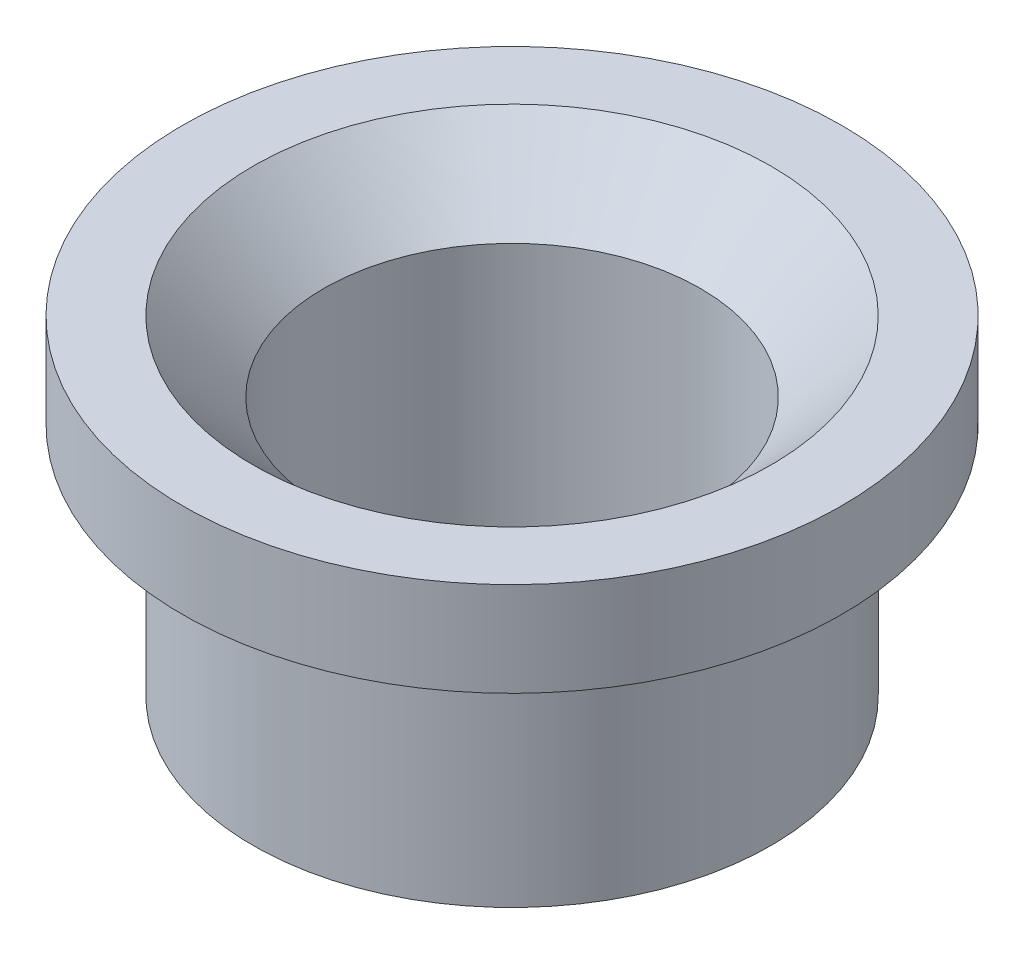
ISO-10303-21;
HEADER;
FILE_DESCRIPTION(('STEP AP214'),'2;1');
FILE_NAME('part.step','',(''),(''),'','','');
FILE_SCHEMA(('AUTOMOTIVE_DESIGN { 1 0 10303 214 1 1 1 1 }'));
ENDSEC;
DATA;
#1=APPLICATION_CONTEXT('core data for automotive mechanical design processes');
#2=APPLICATION_PROTOCOL_DEFINITION('international standard','automotive_design',2000,#1);
#3=PRODUCT_CONTEXT('',#1,'mechanical');
#4=PRODUCT('Part','Part','',(#3));
#5=PRODUCT_RELATED_PRODUCT_CATEGORY('part','',(#4));
#6=PRODUCT_DEFINITION_FORMATION('','',#4);
#7=PRODUCT_DEFINITION_CONTEXT('part definition',#1,'design');
#8=PRODUCT_DEFINITION('design','',#6,#7);
#9=PRODUCT_DEFINITION_SHAPE('','',#8);
#10=(LENGTH_UNIT() NAMED_UNIT(*) SI_UNIT(.MILLI.,.METRE.));
#11=(NAMED_UNIT(*) PLANE_ANGLE_UNIT() SI_UNIT($,.RADIAN.));
#12=(NAMED_UNIT(*) SI_UNIT($,.STERADIAN.) SOLID_ANGLE_UNIT());
#13=UNCERTAINTY_MEASURE_WITH_UNIT(LENGTH_MEASURE(1.E-05),#10,'distance_accuracy_value','');
#14=(GEOMETRIC_REPRESENTATION_CONTEXT(3) GLOBAL_UNCERTAINTY_ASSIGNED_CONTEXT((#13)) GLOBAL_UNIT_ASSIGNED_CONTEXT((#10,
#11,#12)) REPRESENTATION_CONTEXT('',''));
#15=CARTESIAN_POINT('',(0.,0.,0.));
#16=DIRECTION('',(0.,0.,1.));
#17=DIRECTION('',(1.,0.,0.));
#18=AXIS2_PLACEMENT_3D('',#15,#16,#17);
#19=CARTESIAN_POINT('',(16.5,0.,0.));
#20=DIRECTION('',(0.,-1.,0.));
#21=DIRECTION('',(0.,0.,-1.));
#22=AXIS2_PLACEMENT_3D('',#19,#20,#21);
#23=PLANE('',#22);
#24=CARTESIAN_POINT('',(0.,0.,0.));
#25=DIRECTION('',(0.,-1.,0.));
#26=DIRECTION('',(0.,0.,-1.));
#27=AXIS2_PLACEMENT_3D('',#24,#25,#26);
#28=CIRCLE('',#27,16.5);
#29=CARTESIAN_POINT('',(0.,0.,-16.5));
#30=VERTEX_POINT('',#29);
#31=EDGE_CURVE('E65',#30,#30,#28,.T.);
#32=ORIENTED_EDGE('',*,*,#31,.T.);
#33=EDGE_LOOP('',(#32));
#34=FACE_BOUND('',#33,.T.);
#35=CARTESIAN_POINT('',(0.,0.,0.));
#36=DIRECTION('',(0.,-1.,0.));
#37=DIRECTION('',(0.,0.,-1.));
#38=AXIS2_PLACEMENT_3D('',#35,#36,#37);
#39=CIRCLE('',#38,12.);
#40=CARTESIAN_POINT('',(0.,0.,-12.));
#41=VERTEX_POINT('',#40);
#42=EDGE_CURVE('E10',#41,#41,#39,.T.);
#43=ORIENTED_EDGE('',*,*,#42,.F.);
#44=EDGE_LOOP('',(#43));
#45=FACE_BOUND('',#44,.T.);
#46=ADVANCED_FACE('F40',(#34,#45),#23,.T.);
#47=CARTESIAN_POINT('',(0.,0.,0.));
#48=DIRECTION('',(0.,-1.,0.));
#49=DIRECTION('',(0.,0.,-1.));
#50=AXIS2_PLACEMENT_3D('',#47,#48,#49);
#51=CYLINDRICAL_SURFACE('',#50,12.);
#52=ORIENTED_EDGE('',*,*,#42,.T.);
#53=EDGE_LOOP('',(#52));
#54=FACE_BOUND('',#53,.T.);
#55=CARTESIAN_POINT('',(0.,16.5,0.));
#56=DIRECTION('',(0.,-1.,0.));
#57=DIRECTION('',(0.,0.,-1.));
#58=AXIS2_PLACEMENT_3D('',#55,#56,#57);
#59=CIRCLE('',#58,12.);
#60=CARTESIAN_POINT('',(0.,16.5,-12.));
#61=VERTEX_POINT('',#60);
#62=EDGE_CURVE('E43',#61,#61,#59,.T.);
#63=ORIENTED_EDGE('',*,*,#62,.F.);
#64=EDGE_LOOP('',(#63));
#65=FACE_BOUND('',#64,.T.);
#66=ADVANCED_FACE('F78',(#54,#65),#51,.F.);
#67=CARTESIAN_POINT('',(0.,21.,0.));
#68=DIRECTION('',(0.,1.,0.));
#69=DIRECTION('',(0.,0.,1.));
#70=AXIS2_PLACEMENT_3D('',#67,#68,#69);
#71=CONICAL_SURFACE('',#70,16.5,0.785398163397446);
#72=ORIENTED_EDGE('',*,*,#62,.T.);
#73=EDGE_LOOP('',(#72));
#74=FACE_BOUND('',#73,.T.);
#75=CARTESIAN_POINT('',(0.,21.,0.));
#76=DIRECTION('',(0.,-1.,0.));
#77=DIRECTION('',(0.,0.,-1.));
#78=AXIS2_PLACEMENT_3D('',#75,#76,#77);
#79=CIRCLE('',#78,16.5);
#80=CARTESIAN_POINT('',(0.,21.,-16.5));
#81=VERTEX_POINT('',#80);
#82=EDGE_CURVE('E50',#81,#81,#79,.T.);
#83=ORIENTED_EDGE('',*,*,#82,.F.);
#84=EDGE_LOOP('',(#83));
#85=FACE_BOUND('',#84,.T.);
#86=ADVANCED_FACE('F83',(#74,#85),#71,.F.);
#87=CARTESIAN_POINT('',(16.5,21.,0.));
#88=DIRECTION('',(0.,1.,0.));
#89=DIRECTION('',(0.,0.,1.));
#90=AXIS2_PLACEMENT_3D('',#87,#88,#89);
#91=PLANE('',#90);
#92=ORIENTED_EDGE('',*,*,#82,.T.);
#93=EDGE_LOOP('',(#92));
#94=FACE_BOUND('',#93,.T.);
#95=CARTESIAN_POINT('',(0.,21.,0.));
#96=DIRECTION('',(0.,-1.,0.));
#97=DIRECTION('',(0.,0.,-1.));
#98=AXIS2_PLACEMENT_3D('',#95,#96,#97);
#99=CIRCLE('',#98,21.);
#100=CARTESIAN_POINT('',(0.,21.,-21.));
#101=VERTEX_POINT('',#100);
#102=EDGE_CURVE('E51',#101,#101,#99,.T.);
#103=ORIENTED_EDGE('',*,*,#102,.F.);
#104=EDGE_LOOP('',(#103));
#105=FACE_BOUND('',#104,.T.);
#106=ADVANCED_FACE('F86',(#94,#105),#91,.T.);
#107=CARTESIAN_POINT('',(0.,0.,0.));
#108=DIRECTION('',(0.,-1.,0.));
#109=DIRECTION('',(0.,0.,-1.));
#110=AXIS2_PLACEMENT_3D('',#107,#108,#109);
#111=CYLINDRICAL_SURFACE('',#110,21.);
#112=ORIENTED_EDGE('',*,*,#102,.T.);
#113=EDGE_LOOP('',(#112));
#114=FACE_BOUND('',#113,.T.);
#115=CARTESIAN_POINT('',(0.,15.,0.));
#116=DIRECTION('',(0.,-1.,0.));
#117=DIRECTION('',(0.,0.,-1.));
#118=AXIS2_PLACEMENT_3D('',#115,#116,#117);
#119=CIRCLE('',#118,21.);
#120=CARTESIAN_POINT('',(0.,15.,-21.));
#121=VERTEX_POINT('',#120);
#122=EDGE_CURVE('E57',#121,#121,#119,.T.);
#123=ORIENTED_EDGE('',*,*,#122,.F.);
#124=EDGE_LOOP('',(#123));
#125=FACE_BOUND('',#124,.T.);
#126=ADVANCED_FACE('F77',(#114,#125),#111,.T.);
#127=CARTESIAN_POINT('',(21.,15.,0.));
#128=DIRECTION('',(0.,-1.,0.));
#129=DIRECTION('',(0.,0.,-1.));
#130=AXIS2_PLACEMENT_3D('',#127,#128,#129);
#131=PLANE('',#130);
#132=ORIENTED_EDGE('',*,*,#122,.T.);
#133=EDGE_LOOP('',(#132));
#134=FACE_BOUND('',#133,.T.);
#135=CARTESIAN_POINT('',(0.,15.,0.));
#136=DIRECTION('',(0.,-1.,0.));
#137=DIRECTION('',(0.,0.,-1.));
#138=AXIS2_PLACEMENT_3D('',#135,#136,#137);
#139=CIRCLE('',#138,16.5);
#140=CARTESIAN_POINT('',(0.,15.,-16.5));
#141=VERTEX_POINT('',#140);
#142=EDGE_CURVE('E56',#141,#141,#139,.T.);
#143=ORIENTED_EDGE('',*,*,#142,.F.);
#144=EDGE_LOOP('',(#143));
#145=FACE_BOUND('',#144,.T.);
#146=ADVANCED_FACE('F70',(#134,#145),#131,.T.);
#147=CARTESIAN_POINT('',(0.,0.,0.));
#148=DIRECTION('',(0.,-1.,0.));
#149=DIRECTION('',(0.,0.,-1.));
#150=AXIS2_PLACEMENT_3D('',#147,#148,#149);
#151=CYLINDRICAL_SURFACE('',#150,16.5);
#152=ORIENTED_EDGE('',*,*,#142,.T.);
#153=EDGE_LOOP('',(#152));
#154=FACE_BOUND('',#153,.T.);
#155=ORIENTED_EDGE('',*,*,#31,.F.);
#156=EDGE_LOOP('',(#155));
#157=FACE_BOUND('',#156,.T.);
#158=ADVANCED_FACE('F69',(#154,#157),#151,.T.);
#159=CLOSED_SHELL('',(#46,#66,#86,#106,#126,#146,#158));
#160=MANIFOLD_SOLID_BREP('B2',#159);
#161=ADVANCED_BREP_SHAPE_REPRESENTATION('',(#18,#160),#14);
#162=SHAPE_DEFINITION_REPRESENTATION(#9,#161);
ENDSEC;
END-ISO-10303-21;
